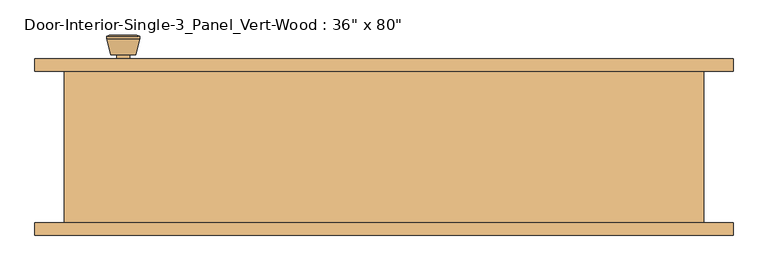
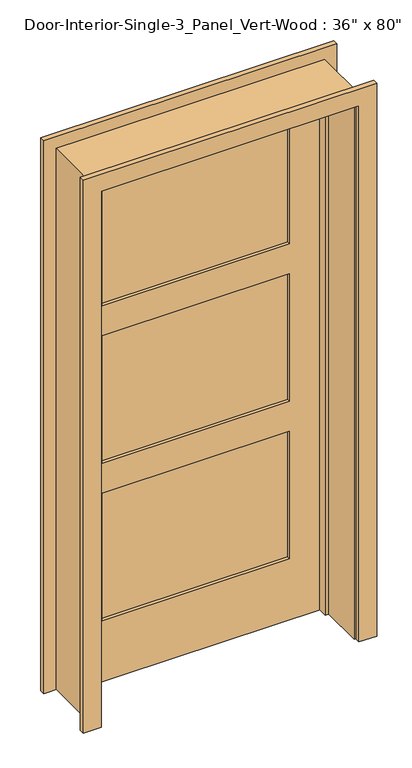
"""IFC4 building model written with IfcOpenShell, lengths in millimetres: door geometry."""

from ifc_helpers import new_model, si_unit, point, frame, frame_2d, origin, place, context, project, spatial, polyline, circle_curve, trimmed, segment, composite_curve, outline, extrude, faceted_brep, source, transform, mapped, element, save
from ifc_brep_helpers import plane_surface, cylinder_surface, revolved_surface, advanced_brep


def door_2334f446(model_context):
    return source(origin(), model_context, "Body", "SolidModel", [
        advanced_brep(
        [(-393.7, 70.2, 914.4), (-383.7, 70.2, 914.4), (-403.7, 70.2, 914.4), (-373.2241324, 21.2, 914.4), (-393.7, 21.2, 914.4), (-414.1758676, 21.2, 914.4), (-368.7, 23.0278681, 914.4), (-418.7, 23.0278681, 914.4), (-368.7, 26.4915463, 914.4), (-418.7, 26.4915463, 914.4), (-375.063764, 51.2, 914.4), (-412.336236, 51.2, 914.4), (-383.7, 51.2, 914.4), (-403.7, 51.2, 914.4)],
        [
            (0, 1),
            (1, 2, circle_curve(frame((-393.7, 70.2, 914.4), z_axis=(0.0, 1.0, 0.0), x_axis=(-1.0, 0.0, 0.0)), 10.0)),
            (2, 0),
            (2, 1, circle_curve(frame((-393.7, 70.2, 914.4), z_axis=(0.0, 1.0, 0.0), x_axis=(-1.0, 0.0, 0.0)), 10.0)),
            (3, 4),
            (4, 5),
            (5, 3, circle_curve(frame((-393.7, 21.2, 914.4), z_axis=(0.0, -1.0, 0.0), x_axis=(-1.0, 0.0, 0.0)), 20.4758676)),
            (3, 5, circle_curve(frame((-393.7, 21.2, 914.4), z_axis=(0.0, -1.0, 0.0), x_axis=(-1.0, 0.0, 0.0)), 20.4758676)),
            (6, 3),
            (5, 7),
            (7, 6, circle_curve(frame((-393.7, 23.0278681, 914.4), z_axis=(0.0, -1.0, 0.0), x_axis=(-1.0, 0.0, 0.0)), 25.0)),
            (6, 7, circle_curve(frame((-393.7, 23.0278681, 914.4), z_axis=(0.0, -1.0, 0.0), x_axis=(-1.0, 0.0, 0.0)), 25.0)),
            (8, 6),
            (7, 9),
            (9, 8, circle_curve(frame((-393.7, 26.4915463, 914.4), z_axis=(0.0, -1.0, 0.0), x_axis=(-1.0, 0.0, 0.0)), 25.0)),
            (8, 9, circle_curve(frame((-393.7, 26.4915463, 914.4), z_axis=(0.0, -1.0, 0.0), x_axis=(-1.0, 0.0, 0.0)), 25.0)),
            (10, 8),
            (9, 11),
            (11, 10, circle_curve(frame((-393.7, 51.2, 914.4), z_axis=(0.0, -1.0, 0.0), x_axis=(-1.0, 0.0, 0.0)), 18.636236)),
            (10, 11, circle_curve(frame((-393.7, 51.2, 914.4), z_axis=(0.0, -1.0, 0.0), x_axis=(-1.0, 0.0, 0.0)), 18.636236)),
            (12, 10),
            (11, 13),
            (13, 12, circle_curve(frame((-393.7, 51.2, 914.4), z_axis=(0.0, -1.0, 0.0), x_axis=(-1.0, 0.0, 0.0)), 10.0)),
            (12, 13, circle_curve(frame((-393.7, 51.2, 914.4), z_axis=(0.0, -1.0, 0.0), x_axis=(-1.0, 0.0, 0.0)), 10.0)),
            (1, 12),
            (13, 2),
        ],
        [
            plane_surface(frame((-393.7, 70.2, 914.4), z_axis=(0.0, 1.0, 0.0), x_axis=(-1.0, 0.0, 0.0))),
            plane_surface(frame((-393.7, 21.2, 914.4), z_axis=(0.0, -1.0, 0.0), x_axis=(-1.0, 0.0, 0.0))),
            revolved_surface(polyline([(-414.1758676, 21.2, 914.4), (-418.7, 23.0278681, 914.4)]), (-393.7, 70.2, 914.4), (0.0, 1.0, 0.0)),
            cylinder_surface(frame((-393.7, 70.2, 914.4), z_axis=(0.0, 1.0, 0.0), x_axis=(-1.0, 0.0, 0.0)), 25.0),
            revolved_surface(polyline([(-418.7, 26.4915463, 914.4), (-412.336236, 51.2, 914.4)]), (-393.7, 70.2, 914.4), (0.0, 1.0, 0.0)),
            plane_surface(frame((-393.7, 51.2, 914.4), z_axis=(0.0, 1.0, 0.0), x_axis=(-1.0, 0.0, 0.0))),
            cylinder_surface(frame((-393.7, 70.2, 914.4), z_axis=(0.0, 1.0, 0.0), x_axis=(-1.0, 0.0, 0.0)), 10.0),
        ],
        [
            (0, [[1, 2, 3]]),
            (0, [[-3, 4, -1]]),
            (1, [[5, 6, 7]]),
            (1, [[-6, -5, 8]]),
            (2, [[9, -7, 10, 11]]),
            (2, [[-10, -8, -9, 12]]),
            (3, [[13, -11, 14, 15]]),
            (3, [[-14, -12, -13, 16]]),
            (4, [[17, -15, 18, 19]]),
            (4, [[-18, -16, -17, 20]]),
            (5, [[21, -19, 22, 23]]),
            (5, [[-22, -20, -21, 24]]),
            (6, [[25, -23, 26, -2]]),
            (6, [[-26, -24, -25, -4]]),
        ],
    ),
        extrude(outline(composite_curve([segment(trimmed(circle_curve(frame_2d((914.4, -393.7)), 30.0), [point((914.4, -423.7))], [point((914.4, -363.7))], False, "CARTESIAN"), True, "CONTINUOUS"), segment(trimmed(circle_curve(frame_2d((914.4, -393.7)), 30.0), [point((914.4, -363.7))], [point((914.4, -423.7))], False, "CARTESIAN"), True, "CONTINUOUS")], self_intersect=False)), frame((0.0, 70.2, 0.0), z_axis=(0.0, 1.0, 0.0), x_axis=(0.0, 0.0, 1.0)), (0.0, 0.0, 1.0), 6.0),
        advanced_brep(
        [(-393.7, 117.125, 914.4), (-403.7, 117.125, 914.4), (-383.7, 117.125, 914.4), (-373.2241324, 166.125, 914.4), (-414.1758676, 166.125, 914.4), (-393.7, 166.125, 914.4), (-368.7, 164.2971319, 914.4), (-418.7, 164.2971319, 914.4), (-368.7, 160.8334537, 914.4), (-418.7, 160.8334537, 914.4), (-375.063764, 136.125, 914.4), (-412.336236, 136.125, 914.4), (-383.7, 136.125, 914.4), (-403.7, 136.125, 914.4)],
        [
            (0, 1),
            (1, 2, circle_curve(frame((-393.7, 117.125, 914.4), z_axis=(0.0, -1.0, 0.0), x_axis=(-1.0, 0.0, 0.0)), 10.0)),
            (2, 0),
            (2, 1, circle_curve(frame((-393.7, 117.125, 914.4), z_axis=(0.0, -1.0, 0.0), x_axis=(-1.0, 0.0, 0.0)), 10.0)),
            (3, 4, circle_curve(frame((-393.7, 166.125, 914.4), z_axis=(0.0, 1.0, 0.0), x_axis=(-1.0, 0.0, 0.0)), 20.4758676)),
            (4, 5),
            (5, 3),
            (4, 3, circle_curve(frame((-393.7, 166.125, 914.4), z_axis=(0.0, 1.0, 0.0), x_axis=(-1.0, 0.0, 0.0)), 20.4758676)),
            (6, 7, circle_curve(frame((-393.7, 164.2971319, 914.4), z_axis=(0.0, 1.0, 0.0), x_axis=(-1.0, 0.0, 0.0)), 25.0)),
            (7, 4),
            (3, 6),
            (7, 6, circle_curve(frame((-393.7, 164.2971319, 914.4), z_axis=(0.0, 1.0, 0.0), x_axis=(-1.0, 0.0, 0.0)), 25.0)),
            (8, 9, circle_curve(frame((-393.7, 160.8334537, 914.4), z_axis=(0.0, 1.0, 0.0), x_axis=(-1.0, 0.0, 0.0)), 25.0)),
            (9, 7),
            (6, 8),
            (9, 8, circle_curve(frame((-393.7, 160.8334537, 914.4), z_axis=(0.0, 1.0, 0.0), x_axis=(-1.0, 0.0, 0.0)), 25.0)),
            (10, 11, circle_curve(frame((-393.7, 136.125, 914.4), z_axis=(0.0, 1.0, 0.0), x_axis=(-1.0, 0.0, 0.0)), 18.636236)),
            (11, 9),
            (8, 10),
            (11, 10, circle_curve(frame((-393.7, 136.125, 914.4), z_axis=(0.0, 1.0, 0.0), x_axis=(-1.0, 0.0, 0.0)), 18.636236)),
            (12, 13, circle_curve(frame((-393.7, 136.125, 914.4), z_axis=(0.0, 1.0, 0.0), x_axis=(-1.0, 0.0, 0.0)), 10.0)),
            (13, 11),
            (10, 12),
            (13, 12, circle_curve(frame((-393.7, 136.125, 914.4), z_axis=(0.0, 1.0, 0.0), x_axis=(-1.0, 0.0, 0.0)), 10.0)),
            (1, 13),
            (12, 2),
        ],
        [
            plane_surface(frame((-393.7, 117.125, 914.4), z_axis=(0.0, -1.0, 0.0), x_axis=(-1.0, 0.0, 0.0))),
            plane_surface(frame((-393.7, 166.125, 914.4), z_axis=(0.0, 1.0, 0.0), x_axis=(-1.0, 0.0, 0.0))),
            revolved_surface(polyline([(-414.1758676, 166.125, 914.4), (-418.7, 164.2971319, 914.4)]), (-393.7, 117.125, 914.4), (0.0, -1.0, 0.0)),
            cylinder_surface(frame((-393.7, 117.125, 914.4), z_axis=(0.0, -1.0, 0.0), x_axis=(-1.0, 0.0, 0.0)), 25.0),
            revolved_surface(polyline([(-418.7, 160.8334537, 914.4), (-412.336236, 136.125, 914.4)]), (-393.7, 117.125, 914.4), (0.0, -1.0, 0.0)),
            plane_surface(frame((-393.7, 136.125, 914.4), z_axis=(0.0, -1.0, 0.0), x_axis=(-1.0, 0.0, 0.0))),
            cylinder_surface(frame((-393.7, 117.125, 914.4), z_axis=(0.0, -1.0, 0.0), x_axis=(-1.0, 0.0, 0.0)), 10.0),
        ],
        [
            (0, [[1, 2, 3]]),
            (0, [[-3, 4, -1]]),
            (1, [[5, 6, 7]]),
            (1, [[8, -7, -6]]),
            (2, [[9, 10, -5, 11]]),
            (2, [[12, -11, -8, -10]]),
            (3, [[13, 14, -9, 15]]),
            (3, [[16, -15, -12, -14]]),
            (4, [[17, 18, -13, 19]]),
            (4, [[20, -19, -16, -18]]),
            (5, [[21, 22, -17, 23]]),
            (5, [[24, -23, -20, -22]]),
            (6, [[-2, 25, -21, 26]]),
            (6, [[-4, -26, -24, -25]]),
        ],
    ),
        extrude(outline(composite_curve([segment(trimmed(circle_curve(frame_2d((914.4, -393.7)), 30.0), [point((914.4, -423.7))], [point((914.4, -363.7))], False, "CARTESIAN"), True, "CONTINUOUS"), segment(trimmed(circle_curve(frame_2d((914.4, -393.7)), 30.0), [point((914.4, -363.7))], [point((914.4, -423.7))], False, "CARTESIAN"), True, "CONTINUOUS")], self_intersect=False)), frame((0.0, 111.125, 0.0), z_axis=(0.0, 1.0, 0.0), x_axis=(0.0, 0.0, 1.0)), (0.0, 0.0, 1.0), 6.0),
        faceted_brep([(482.6, 111.125, 0.0), (482.6, -117.475, 0.0), (457.2, -117.475, 0.0), (457.2, 41.275, 0.0), (444.5, 41.275, 0.0), (444.5, 76.2, 0.0), (457.2, 76.2, 0.0), (457.2, 111.125, 0.0), (482.6, 111.125, 2057.4), (482.6, -117.475, 2057.4), (-482.6, -117.475, 2057.4), (-482.6, -117.475, 0.0), (-457.2, -117.475, 0.0), (-457.2, -117.475, 2032.0), (457.2, -117.475, 2032.0), (457.2, 41.275, 2032.0), (-457.2, 41.275, 2032.0), (-457.2, 41.275, 0.0), (-444.5, 41.275, 0.0), (-444.5, 41.275, 2019.3), (444.5, 41.275, 2019.3), (444.5, 76.2, 2019.3), (-444.5, 76.2, 2019.3), (-444.5, 76.2, 0.0), (-457.2, 76.2, 0.0), (-457.2, 76.2, 2032.0), (457.2, 76.2, 2032.0), (457.2, 111.125, 2032.0), (-457.2, 111.125, 2032.0), (-457.2, 111.125, 0.0), (-482.6, 111.125, 0.0), (-482.6, 111.125, 2057.4)], [[[0, 1, 2, 3, 4, 5, 6, 7]], [[1, 0, 8, 9]], [[2, 1, 9, 10, 11, 12, 13, 14]], [[3, 2, 14, 15]], [[4, 3, 15, 16, 17, 18, 19, 20]], [[5, 4, 20, 21]], [[6, 5, 21, 22, 23, 24, 25, 26]], [[7, 6, 26, 27]], [[0, 7, 27, 28, 29, 30, 31, 8]], [[9, 8, 31, 10]], [[15, 14, 13, 16]], [[21, 20, 19, 22]], [[27, 26, 25, 28]], [[30, 29, 24, 23, 18, 17, 12, 11]], [[10, 31, 30, 11]], [[16, 13, 12, 17]], [[22, 19, 18, 23]], [[28, 25, 24, 29]]]),
        extrude(outline(polyline([(2032.0, -457.2), (0.0, -457.2), (0.0, 457.2), (2032.0, 457.2), (2032.0, -457.2)]), holes=[polyline([(1912.9375, -336.55), (1912.9375, 336.55), (1428.75, 336.55), (1428.75, -336.55), (1912.9375, -336.55)]), polyline([(715.9625, -336.55), (715.9625, 336.55), (231.775, 336.55), (231.775, -336.55), (715.9625, -336.55)]), polyline([(1314.45, -336.55), (1314.45, 336.55), (830.2625, 336.55), (830.2625, -336.55), (1314.45, -336.55)])]), frame((0.0, 76.2, 0.0), z_axis=(0.0, 1.0, 0.0), x_axis=(0.0, 0.0, 1.0)), (0.0, 0.0, 1.0), 34.925),
        extrude(outline(polyline([(336.55, 87.8416667), (-336.55, 87.8416667), (-336.55, 99.4833333), (336.55, 99.4833333), (336.55, 87.8416667)])), frame((0.0, 0.0, 1428.75), z_axis=(0.0, 0.0, 1.0), x_axis=(1.0, 0.0, 0.0)), (0.0, 0.0, 1.0), 484.1875),
        extrude(outline(polyline([(336.55, 87.8416667), (-336.55, 87.8416667), (-336.55, 99.4833333), (336.55, 99.4833333), (336.55, 87.8416667)])), frame((0.0, 0.0, 231.775), z_axis=(0.0, 0.0, 1.0), x_axis=(1.0, 0.0, 0.0)), (0.0, 0.0, 1.0), 484.1875),
        extrude(outline(polyline([(336.55, 87.8416667), (-336.55, 87.8416667), (-336.55, 99.4833333), (336.55, 99.4833333), (336.55, 87.8416667)])), frame((0.0, 0.0, 830.2625), z_axis=(0.0, 0.0, 1.0), x_axis=(1.0, 0.0, 0.0)), (0.0, 0.0, 1.0), 484.1875),
        extrude(outline(polyline([(0.0, 463.55), (0.0, 527.05), (2101.85, 527.05), (2101.85, -527.05), (0.0, -527.05), (0.0, -463.55), (2038.35, -463.55), (2038.35, 463.55), (0.0, 463.55)])), frame((0.0, 111.125, 0.0), z_axis=(0.0, 1.0, 0.0), x_axis=(0.0, 0.0, 1.0)), (0.0, 0.0, 1.0), 19.05),
        extrude(outline(polyline([(0.0, 463.55), (0.0, 527.05), (2101.85, 527.05), (2101.85, -527.05), (0.0, -527.05), (0.0, -463.55), (2038.35, -463.55), (2038.35, 463.55), (0.0, 463.55)])), frame((0.0, -136.525, 0.0), z_axis=(0.0, 1.0, 0.0), x_axis=(0.0, 0.0, 1.0)), (0.0, 0.0, 1.0), 19.05),
    ])


if __name__ == "__main__":
    model = new_model("IFC4")
    model_context = context("Model", 3, world=origin())
    ifc_project = project(units=[si_unit("LENGTHUNIT", "METRE", prefix="MILLI")], contexts=[model_context])
    site = spatial("IfcSite", under=ifc_project)
    building = spatial("IfcBuilding", under=site)
    placement = place(None, origin())
    door_shape = door_2334f446(model_context)
    element("IfcDoor", 1, ObjectType="Door-Interior-Single-3_Panel_Vert-Wood : 36\" x 80\"", at=placement, inside=building, context=model_context, shape_type="MappedRepresentation", body=[
        mapped(door_shape, transform((0.0, 0.0, 0.0), x_axis=(1.0, 0.0, 0.0), y_axis=(0.0, 1.0, 0.0), z_axis=(0.0, 0.0, 1.0))),
    ])
    save(model, "model.ifc")

# Revit data of these elements
# Type "Door-Interior-Single-3_Panel_Vert-Wood : 36\" x 80\""
#   Type Mark = "10"
#   Assembly Code = "C1020300"
#   Analytic Construction = "Wooden"
#   Top Rail = 0' - 4 11/16"
#   Thickness = 0' - 1 3/8"
#   Thermal Resistance (R) = 2.5876 (h·ft²·°F)/BTU
#   Swing Angle [instance default] = 90.00°
#   Stiles = 0' - 4 3/4"
#   Rough Width = 3' - 2"
#   Rough Height = 6' - 9"
#   Intermediate Rail = 0' - 4 1/2"
#   Height = 6' - 8"
#   Width = 3' - 0"
#   Heat Transfer Coefficient (U) = 0.3865 BTU/(h·ft²·°F)
#   Bottom Rail = 0' - 9 1/8"
#   Trim Material = Cherry
#   Panel Material = Cherry
#   Frame Material = Cherry
#   Door Handle Material = Aluminum
#   Visual Light Transmittance = 0
#   Solar Heat Gain Coefficient = 0
#   Wall Closure = (empty or 0)
#   Function = (empty or 0)
# Element 1 (IfcDoor, "Door-Interior-Single-3_Panel_Vert-Wood : 36\" x 80\"")
#   Materials on its faces: "Cherry", "Aluminum"
# Materials
#   "Cherry": class "Wood", colour RGB 226 177 128, transparency 0, Description = "Prunus Serotina", Cost = 0
#   "Aluminum": class "Metal", colour RGB 247 247 247, transparency 0, Description = "Aluminum 6061", Cost = 0
